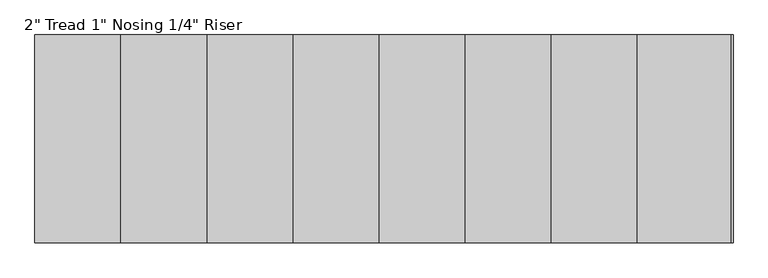
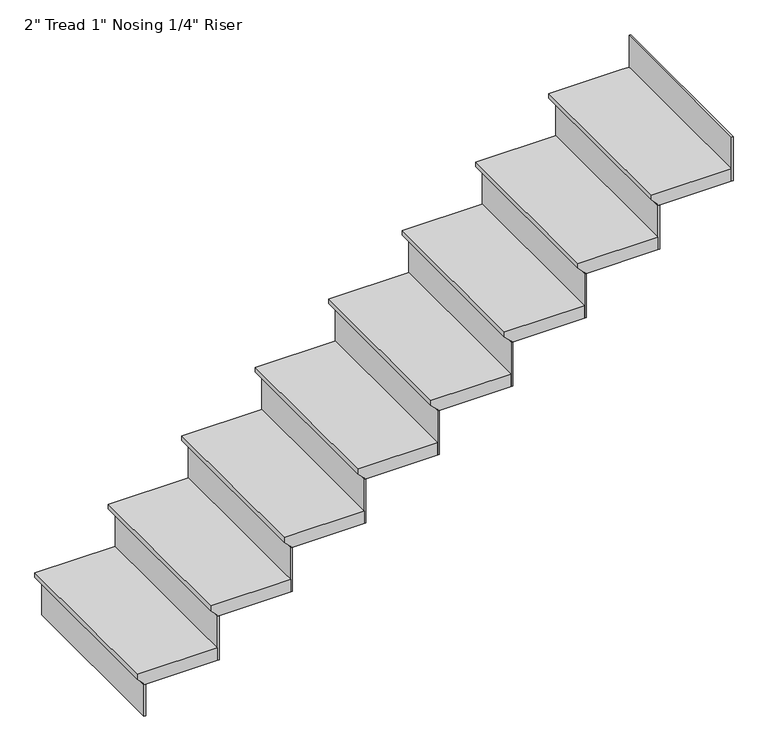
"""IFC4 building model written with IfcOpenShell, lengths in millimetres: stair flight geometry."""

from ifc_helpers import new_model, si_unit, origin, place, context, project, spatial, faceted_brep, source, transform, mapped, element, save


def stair_flight_99ccf548(model_context):
    return source(origin(), model_context, "Body", "Brep", [
        faceted_brep([(-5185.8837185, -7060.9366292, 158.75), (-5185.8837185, -7060.9366292, 177.8), (-5185.8837185, -6386.6877785, 177.8), (-5185.8837185, -6386.6877785, 158.75), (-5160.4837185, -7060.9366292, 133.35), (-5160.4837185, -6386.6877785, 133.35), (-4881.0837185, -7060.9366292, 177.8), (-4881.0837185, -6386.6877785, 177.8), (-5160.4837185, -6386.6877785, 127.0), (-4881.0837185, -6386.6877785, 127.0), (-4881.0837185, -7060.9366292, 127.0), (-5160.4837185, -7060.9366292, 127.0)], [[[0, 1, 2, 3]], [[4, 0, 3, 5]], [[2, 1, 6, 7]], [[8, 9, 10, 11]], [[2, 7, 9, 8, 5, 3]], [[8, 11, 4, 5]], [[6, 1, 0, 4, 11, 10]], [[7, 6, 10, 9]]]),
        faceted_brep([(-5160.4837185, -7060.9366292, 127.0), (-5160.4837185, -7060.9366292, 0.0), (-5154.1337185, -7060.9366292, 0.0), (-5154.1337185, -7060.9366292, 127.0), (-5160.4837185, -6386.6877785, 127.0), (-5154.1337185, -6386.6877785, 127.0), (-5154.1337185, -6386.6877785, 0.0), (-5160.4837185, -6386.6877785, 0.0)], [[[0, 1, 2, 3]], [[4, 5, 6, 7]], [[1, 0, 4, 7]], [[2, 1, 7, 6]], [[3, 2, 6, 5]], [[0, 3, 5, 4]]]),
        faceted_brep([(-4881.0837185, -7060.9366292, 304.8), (-4881.0837185, -7060.9366292, 127.0), (-4874.7337185, -7060.9366292, 127.0), (-4874.7337185, -7060.9366292, 304.8), (-4881.0837185, -6386.6877785, 304.8), (-4874.7337185, -6386.6877785, 304.8), (-4874.7337185, -6386.6877785, 127.0), (-4881.0837185, -6386.6877785, 127.0)], [[[0, 1, 2, 3]], [[4, 5, 6, 7]], [[1, 0, 4, 7]], [[2, 1, 7, 6]], [[3, 2, 6, 5]], [[0, 3, 5, 4]]]),
        faceted_brep([(-4906.4837185, -6386.6877785, 355.6), (-4906.4837185, -7060.9366292, 355.6), (-4601.6837185, -7060.9366292, 355.6), (-4601.6837185, -6386.6877785, 355.6), (-4881.0837185, -6386.6877785, 304.8), (-4601.6837185, -6386.6877785, 304.8), (-4601.6837185, -7060.9366292, 304.8), (-4881.0837185, -7060.9366292, 304.8), (-4881.0837185, -6386.6877785, 311.15), (-4906.4837185, -6386.6877785, 336.55), (-4881.0837185, -7060.9366292, 311.15), (-4906.4837185, -7060.9366292, 336.55)], [[[0, 1, 2, 3]], [[4, 5, 6, 7]], [[0, 3, 5, 4, 8, 9]], [[4, 7, 10, 8]], [[2, 1, 11, 10, 7, 6]], [[3, 2, 6, 5]], [[11, 1, 0, 9]], [[10, 11, 9, 8]]]),
        faceted_brep([(-4601.6837185, -7060.9366292, 482.6), (-4601.6837185, -7060.9366292, 304.8), (-4595.3337185, -7060.9366292, 304.8), (-4595.3337185, -7060.9366292, 482.6), (-4601.6837185, -6386.6877785, 482.6), (-4595.3337185, -6386.6877785, 482.6), (-4595.3337185, -6386.6877785, 304.8), (-4601.6837185, -6386.6877785, 304.8)], [[[0, 1, 2, 3]], [[4, 5, 6, 7]], [[1, 0, 4, 7]], [[2, 1, 7, 6]], [[3, 2, 6, 5]], [[0, 3, 5, 4]]]),
        faceted_brep([(-4627.0837185, -6386.6877785, 533.4), (-4627.0837185, -7060.9366292, 533.4), (-4322.2837185, -7060.9366292, 533.4), (-4322.2837185, -6386.6877785, 533.4), (-4601.6837185, -6386.6877785, 482.6), (-4322.2837185, -6386.6877785, 482.6), (-4322.2837185, -7060.9366292, 482.6), (-4601.6837185, -7060.9366292, 482.6), (-4601.6837185, -6386.6877785, 488.95), (-4627.0837185, -6386.6877785, 514.35), (-4601.6837185, -7060.9366292, 488.95), (-4627.0837185, -7060.9366292, 514.35)], [[[0, 1, 2, 3]], [[4, 5, 6, 7]], [[0, 3, 5, 4, 8, 9]], [[4, 7, 10, 8]], [[2, 1, 11, 10, 7, 6]], [[3, 2, 6, 5]], [[11, 1, 0, 9]], [[10, 11, 9, 8]]]),
        faceted_brep([(-4322.2837185, -7060.9366292, 660.4), (-4322.2837185, -7060.9366292, 482.6), (-4315.9337185, -7060.9366292, 482.6), (-4315.9337185, -7060.9366292, 660.4), (-4322.2837185, -6386.6877785, 660.4), (-4315.9337185, -6386.6877785, 660.4), (-4315.9337185, -6386.6877785, 482.6), (-4322.2837185, -6386.6877785, 482.6)], [[[0, 1, 2, 3]], [[4, 5, 6, 7]], [[1, 0, 4, 7]], [[2, 1, 7, 6]], [[3, 2, 6, 5]], [[0, 3, 5, 4]]]),
        faceted_brep([(-4347.6837185, -6386.6877785, 711.2), (-4347.6837185, -7060.9366292, 711.2), (-4042.8837185, -7060.9366292, 711.2), (-4042.8837185, -6386.6877785, 711.2), (-4322.2837185, -6386.6877785, 660.4), (-4042.8837185, -6386.6877785, 660.4), (-4042.8837185, -7060.9366292, 660.4), (-4322.2837185, -7060.9366292, 660.4), (-4322.2837185, -6386.6877785, 666.75), (-4347.6837185, -6386.6877785, 692.15), (-4322.2837185, -7060.9366292, 666.75), (-4347.6837185, -7060.9366292, 692.15)], [[[0, 1, 2, 3]], [[4, 5, 6, 7]], [[0, 3, 5, 4, 8, 9]], [[4, 7, 10, 8]], [[2, 1, 11, 10, 7, 6]], [[3, 2, 6, 5]], [[11, 1, 0, 9]], [[10, 11, 9, 8]]]),
        faceted_brep([(-4042.8837185, -7060.9366292, 838.2), (-4042.8837185, -7060.9366292, 660.4), (-4036.5337185, -7060.9366292, 660.4), (-4036.5337185, -7060.9366292, 838.2), (-4042.8837185, -6386.6877785, 838.2), (-4036.5337185, -6386.6877785, 838.2), (-4036.5337185, -6386.6877785, 660.4), (-4042.8837185, -6386.6877785, 660.4)], [[[0, 1, 2, 3]], [[4, 5, 6, 7]], [[1, 0, 4, 7]], [[2, 1, 7, 6]], [[3, 2, 6, 5]], [[0, 3, 5, 4]]]),
        faceted_brep([(-4068.2837185, -6386.6877785, 889.0), (-4068.2837185, -7060.9366292, 889.0), (-3763.4837185, -7060.9366292, 889.0), (-3763.4837185, -6386.6877785, 889.0), (-4042.8837185, -6386.6877785, 838.2), (-3763.4837185, -6386.6877785, 838.2), (-3763.4837185, -7060.9366292, 838.2), (-4042.8837185, -7060.9366292, 838.2), (-4042.8837185, -6386.6877785, 844.55), (-4068.2837185, -6386.6877785, 869.95), (-4042.8837185, -7060.9366292, 844.55), (-4068.2837185, -7060.9366292, 869.95)], [[[0, 1, 2, 3]], [[4, 5, 6, 7]], [[0, 3, 5, 4, 8, 9]], [[4, 7, 10, 8]], [[2, 1, 11, 10, 7, 6]], [[3, 2, 6, 5]], [[11, 1, 0, 9]], [[10, 11, 9, 8]]]),
        faceted_brep([(-3763.4837185, -7060.9366292, 1016.0), (-3763.4837185, -7060.9366292, 838.2), (-3757.1337185, -7060.9366292, 838.2), (-3757.1337185, -7060.9366292, 1016.0), (-3763.4837185, -6386.6877785, 1016.0), (-3757.1337185, -6386.6877785, 1016.0), (-3757.1337185, -6386.6877785, 838.2), (-3763.4837185, -6386.6877785, 838.2)], [[[0, 1, 2, 3]], [[4, 5, 6, 7]], [[1, 0, 4, 7]], [[2, 1, 7, 6]], [[3, 2, 6, 5]], [[0, 3, 5, 4]]]),
        faceted_brep([(-3788.8837185, -6386.6877785, 1066.8), (-3788.8837185, -7060.9366292, 1066.8), (-3484.0837185, -7060.9366292, 1066.8), (-3484.0837185, -6386.6877785, 1066.8), (-3763.4837185, -6386.6877785, 1016.0), (-3484.0837185, -6386.6877785, 1016.0), (-3484.0837185, -7060.9366292, 1016.0), (-3763.4837185, -7060.9366292, 1016.0), (-3763.4837185, -6386.6877785, 1022.35), (-3788.8837185, -6386.6877785, 1047.75), (-3763.4837185, -7060.9366292, 1022.35), (-3788.8837185, -7060.9366292, 1047.75)], [[[0, 1, 2, 3]], [[4, 5, 6, 7]], [[0, 3, 5, 4, 8, 9]], [[4, 7, 10, 8]], [[2, 1, 11, 10, 7, 6]], [[3, 2, 6, 5]], [[11, 1, 0, 9]], [[10, 11, 9, 8]]]),
        faceted_brep([(-3484.0837185, -7060.9366292, 1193.8), (-3484.0837185, -7060.9366292, 1016.0), (-3477.7337185, -7060.9366292, 1016.0), (-3477.7337185, -7060.9366292, 1193.8), (-3484.0837185, -6386.6877785, 1193.8), (-3477.7337185, -6386.6877785, 1193.8), (-3477.7337185, -6386.6877785, 1016.0), (-3484.0837185, -6386.6877785, 1016.0)], [[[0, 1, 2, 3]], [[4, 5, 6, 7]], [[1, 0, 4, 7]], [[2, 1, 7, 6]], [[3, 2, 6, 5]], [[0, 3, 5, 4]]]),
        faceted_brep([(-3509.4837185, -6386.6877785, 1244.6), (-3509.4837185, -7060.9366292, 1244.6), (-3204.6837185, -7060.9366292, 1244.6), (-3204.6837185, -6386.6877785, 1244.6), (-3484.0837185, -6386.6877785, 1193.8), (-3204.6837185, -6386.6877785, 1193.8), (-3204.6837185, -7060.9366292, 1193.8), (-3484.0837185, -7060.9366292, 1193.8), (-3484.0837185, -6386.6877785, 1200.15), (-3509.4837185, -6386.6877785, 1225.55), (-3484.0837185, -7060.9366292, 1200.15), (-3509.4837185, -7060.9366292, 1225.55)], [[[0, 1, 2, 3]], [[4, 5, 6, 7]], [[0, 3, 5, 4, 8, 9]], [[4, 7, 10, 8]], [[2, 1, 11, 10, 7, 6]], [[3, 2, 6, 5]], [[11, 1, 0, 9]], [[10, 11, 9, 8]]]),
        faceted_brep([(-2925.2837185, -7060.9366292, 1549.4), (-2925.2837185, -7060.9366292, 1371.6), (-2918.9337185, -7060.9366292, 1371.6), (-2918.9337185, -7060.9366292, 1549.4), (-2925.2837185, -6386.6877785, 1549.4), (-2918.9337185, -6386.6877785, 1549.4), (-2918.9337185, -6386.6877785, 1371.6), (-2925.2837185, -6386.6877785, 1371.6)], [[[0, 1, 2, 3]], [[4, 5, 6, 7]], [[1, 0, 4, 7]], [[2, 1, 7, 6]], [[3, 2, 6, 5]], [[0, 3, 5, 4]]]),
        faceted_brep([(-3204.6837185, -7060.9366292, 1371.6), (-3204.6837185, -7060.9366292, 1193.8), (-3198.3337185, -7060.9366292, 1193.8), (-3198.3337185, -7060.9366292, 1371.6), (-3204.6837185, -6386.6877785, 1371.6), (-3198.3337185, -6386.6877785, 1371.6), (-3198.3337185, -6386.6877785, 1193.8), (-3204.6837185, -6386.6877785, 1193.8)], [[[0, 1, 2, 3]], [[4, 5, 6, 7]], [[1, 0, 4, 7]], [[2, 1, 7, 6]], [[3, 2, 6, 5]], [[0, 3, 5, 4]]]),
        faceted_brep([(-2925.2837185, -6386.6877785, 1422.4), (-2950.6837185, -6386.6877785, 1422.4), (-3230.0837185, -6386.6877785, 1422.4), (-3230.0837185, -7060.9366292, 1422.4), (-2925.2837185, -7060.9366292, 1422.4), (-2950.6837185, -6386.6877785, 1371.6), (-2925.2837185, -6386.6877785, 1371.6), (-2925.2837185, -7060.9366292, 1371.6), (-3204.6837185, -7060.9366292, 1371.6), (-3204.6837185, -6386.6877785, 1371.6), (-3204.6837185, -6386.6877785, 1377.95), (-3230.0837185, -6386.6877785, 1403.35), (-3204.6837185, -7060.9366292, 1377.95), (-3230.0837185, -7060.9366292, 1403.35)], [[[0, 1, 2, 3, 4]], [[5, 6, 7, 8, 9]], [[1, 0, 6, 5]], [[2, 1, 5, 9, 10, 11]], [[9, 8, 12, 10]], [[4, 3, 13, 12, 8, 7]], [[0, 4, 7, 6]], [[13, 3, 2, 11]], [[12, 13, 11, 10]]]),
    ])


if __name__ == "__main__":
    model = new_model("IFC4")
    model_context = context("Model", 3, world=origin())
    ifc_project = project(units=[si_unit("LENGTHUNIT", "METRE", prefix="MILLI")], contexts=[model_context])
    site = spatial("IfcSite", under=ifc_project)
    building = spatial("IfcBuilding", under=site)
    placement = place(None, origin())
    stair_flight_shape = stair_flight_99ccf548(model_context)
    element("IfcStairFlight", 1, ObjectType="2\" Tread 1\" Nosing 1/4\" Riser", at=placement, inside=building, context=model_context, shape_type="MappedRepresentation", body=[
        mapped(stair_flight_shape, transform((0.0, 0.0, 0.0), x_axis=(1.0, 0.0, 0.0), y_axis=(0.0, 1.0, 0.0), z_axis=(0.0, 0.0, 1.0))),
    ])
    save(model, "model.ifc")
